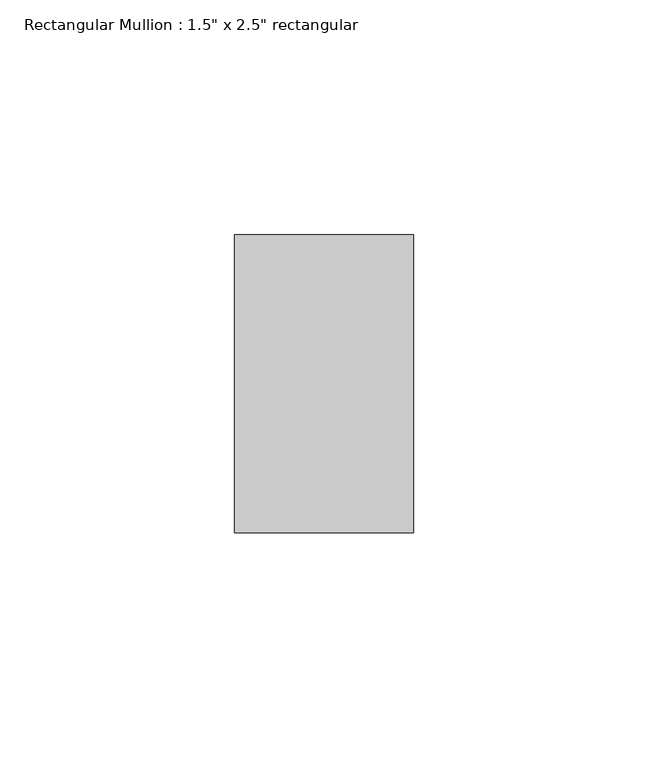
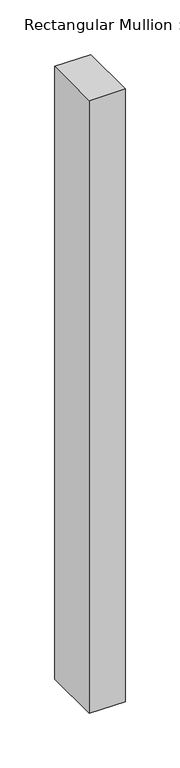
"""IFC4 building model written with IfcOpenShell, lengths in millimetres: member geometry."""

from ifc_helpers import new_model, si_unit, frame, origin, place, context, project, spatial, polyline, outline, extrude, source, transform, mapped, element, save


def member_6458fcce(model_context):
    return source(origin(), model_context, "Body", "SweptSolid", [
        extrude(outline(polyline([(19.05, 31.75), (19.05, -31.75), (-19.05, -31.75), (-19.05, 31.75), (19.05, 31.75)])), frame((0.0, 0.0, -685.8), z_axis=(0.0, 0.0, 1.0), x_axis=(1.0, 0.0, 0.0)), (0.0, 0.0, 1.0), 685.8),
    ])


if __name__ == "__main__":
    model = new_model("IFC4")
    model_context = context("Model", 3, world=origin())
    ifc_project = project(units=[si_unit("LENGTHUNIT", "METRE", prefix="MILLI")], contexts=[model_context])
    site = spatial("IfcSite", under=ifc_project)
    building = spatial("IfcBuilding", under=site)
    placement = place(None, origin())
    member_shape = member_6458fcce(model_context)
    element("IfcMember", 1, ObjectType="Rectangular Mullion : 1.5\" x 2.5\" rectangular", at=placement, inside=building, context=model_context, shape_type="MappedRepresentation", body=[
        mapped(member_shape, transform((0.0, 0.0, 0.0), x_axis=(1.0, 0.0, 0.0), y_axis=(0.0, 1.0, 0.0), z_axis=(0.0, 0.0, 1.0))),
    ])
    save(model, "model.ifc")

# Revit data of these elements
# Type "Rectangular Mullion : 1.5\" x 2.5\" rectangular"
#   built-in parameter 1007304 = 0.208333 (stored number, unit not read)
#   built-in parameter 1007301 = 0.0625 (stored number, unit not read)
#   built-in parameter 1007300 = 0.0625 (stored number, unit not read)
